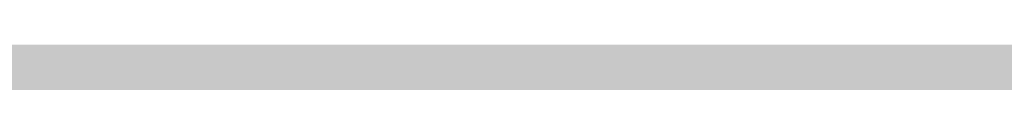
# Model space of a CAD drawing. Units: feet. Extents: x 3168 to 4724, y 827 to 1477.
# Tile 196 of 256: x 3316.07 to 3333.46, y 1098.34 to 1099. Entities that reach past the tile are written whole.
import ezdxf

# ---------------------------------------------------------------- set-up
doc = ezdxf.new("R2010")
doc.units = ezdxf.units.FT
doc.layers.add('A-ELEV', color=7, linetype='Continuous', lineweight=35)
doc.layers.add('A-ELEV-PATT', color=8, linetype='Continuous', lineweight=13)

msp = doc.modelspace()

# ---------------------------------------------------------------- hatches: boundary and pattern name
at = {"layer": 'A-ELEV-PATT'}
h = msp.add_hatch(color=256, dxfattribs=at)
h.dxf.hatch_style = 1
edge = h.paths.add_edge_path()
edge.add_ellipse((3552.906, 979.22), major_axis=(36.745, 0), ratio=0.484848, start_angle=0, end_angle=360)
edge = h.paths.add_edge_path()
edge.add_ellipse((3559.892, 929.252), major_axis=(36.745, 0), ratio=0.484848, start_angle=0, end_angle=360)
edge = h.paths.add_edge_path()
edge.add_line((3299.317, 1198.606), (3479.917, 1198.606))
edge.add_line((3479.917, 1198.606), (3479.917, 1209.869))
edge.add_spline(control_points=[(3479.917, 1209.869), (3464.301, 1209.869), (3448.686, 1209.869), (3410.949, 1209.869), (3388.828, 1209.869), (3355.647, 1209.869), (3344.586, 1209.869), (3327.996, 1209.869), (3322.466, 1209.869), (3314.17, 1209.869), (3311.405, 1209.869), (3307.257, 1209.869), (3305.875, 1209.869), (3303.801, 1209.869), (3303.11, 1209.869), (3302.073, 1209.869), (3301.727, 1209.869), (3301.209, 1209.869), (3301.036, 1209.869), (3300.777, 1209.869), (3300.69, 1209.869), (3300.561, 1209.869), (3300.517, 1209.869), (3300.453, 1209.869), (3300.431, 1209.869), (3300.399, 1209.869), (3300.388, 1209.869), (3300.366, 1209.869), (3300.346, 1209.869), (3300.346, 1209.869), (3300.346, 1209.869), (3300.343, 1209.869), (3300.341, 1209.869), (3300.338, 1209.869), (3300.337, 1209.869), (3300.334, 1209.869), (3300.332, 1209.869), (3300.326, 1209.869), (3300.321, 1209.869), (3300.311, 1209.869), (3300.306, 1209.869), (3300.291, 1209.869), (3300.28, 1209.869), (3300.232, 1209.869), (3300.195, 1209.869), (3299.951, 1209.871), (3299.745, 1209.874), (3299.437, 1209.883), (3299.334, 1209.887), (3299.181, 1209.893), (3299.13, 1209.895), (3298.652, 1209.917), (3298.229, 1209.946), (3297.602, 1210.002), (3297.393, 1210.023), (3297.083, 1210.058), (3296.979, 1210.07), (3296.293, 1210.155), (3295.718, 1210.243), (3294.869, 1210.399), (3294.588, 1210.454), (3294.169, 1210.543), (3294.03, 1210.574), (3291.707, 1211.101), (3289.654, 1211.813), (3285.776, 1213.564), (3283.951, 1214.603), (3280.512, 1216.98), (3278.897, 1218.318), (3276.38, 1220.829), (3275.416, 1221.918), (3274.039, 1223.708), (3273.581, 1224.35), (3273.143, 1225.016)], knot_values=[39.119033, 39.119033, 39.119033, 39.119033, 39.286353, 39.286353, 39.523379, 39.523379, 39.641892, 39.641892, 39.701148, 39.701148, 39.730777, 39.730777, 39.745591, 39.745591, 39.752998, 39.752998, 39.756701, 39.756701, 39.758553, 39.758553, 39.759479, 39.759479, 39.759942, 39.759942, 39.760173, 39.760173, 39.760289, 39.760289, 39.760405, 39.760405, 39.760463, 39.760463, 39.763389, 39.763389, 39.764851, 39.764851, 39.767304, 39.767304, 39.773825, 39.773825, 39.78057, 39.78057, 39.79477, 39.79477, 39.845194, 39.845194, 40.126715, 40.126715, 40.267476, 40.267476, 40.337856, 40.337856, 40.927023, 40.927023, 41.221606, 41.221606, 41.368898, 41.368898, 42.202622, 42.202622, 42.619485, 42.619485, 42.827916, 42.827916, 46.118323, 46.118323, 49.408731, 49.408731, 52.699139, 52.699139, 54.927489, 54.927489, 56.104228, 56.104228, 56.104228, 56.104228], weights=[1, 1, 1, 1, 1, 1, 1, 1, 1, 1, 1, 1, 1, 1, 1, 1, 1, 1, 1, 1, 1, 1, 1, 1, 1, 1, 1, 1, 1, 1, 1, 1, 1, 1, 1, 1, 1, 1, 1, 1, 1, 1, 1, 1, 1, 1, 1, 1, 1, 1, 1, 1, 1, 1, 1, 1, 1, 1, 1, 1, 1, 1, 1, 1, 1, 1, 1, 1, 1, 1, 1, 1, 1, 1], degree=3, periodic=0)
edge.add_line((3273.143, 1225.016), (3273.143, 1099.016))
edge.add_line((3273.143, 1099.016), (3299.317, 1099.016))
edge.add_line((3299.317, 1099.016), (3299.317, 1198.606))
edge = h.paths.add_edge_path()
edge.add_line((3304.758, 1324.158), (3479.917, 1324.158))
edge.add_line((3479.917, 1324.158), (3479.917, 1335.715))
edge.add_line((3479.917, 1335.715), (3269.162, 1335.715))
edge.add_spline(control_points=[(3269.162, 1335.715), (3264.024, 1335.715), (3258.364, 1328.958), (3259.264, 1323.9)], knot_values=[0, 0, 0, 0, 15.412191, 15.412191, 15.412191, 15.412191], degree=3, periodic=0)
edge.add_line((3259.264, 1323.9), (3265.517, 1288.769))
edge.add_line((3265.517, 1288.769), (3275.265, 1261.546))
edge.add_line((3275.265, 1261.546), (3304.758, 1261.546))
edge.add_line((3304.758, 1261.546), (3304.758, 1324.158))
h = msp.add_hatch(color=256, dxfattribs=at)
h.dxf.hatch_style = 1
h.paths.add_polyline_path([(3384.525, 1099.016), (3335.029, 1099.016), (3299.317, 1099.016), (3273.143, 1099.016), (3217.565, 1099.016), (3168.069, 827.116), (3335.029, 827.116)])

# ---------------------------------------------------------------- linework, layer by layer
at = {"layer": 'A-ELEV'}
msp.add_open_spline([(3808.52, 1099.016), (3808.52, 1141.413), (3808.52, 1183.81), (3808.52, 1226.635), (3808.52, 1227.064), (3808.52, 1227.492), (3811.492, 1248.995), (3814.464, 1270.498), (3817.465, 1292.218), (3817.495, 1292.435), (3817.525, 1292.652), (3817.573, 1310.107), (3817.62, 1327.562), (3817.668, 1345.016), (3817.668, 1345.458), (3817.668, 1345.9), (3817.668, 1346.456), (3817.668, 1346.571), (3817.668, 1346.753), (3817.668, 1346.82), (3817.668, 1346.935), (3817.668, 1346.982), (3817.668, 1347.039), (3817.668, 1347.047), (3817.668, 1347.074), (3817.668, 1347.059), (3817.668, 1347.062), (3817.668, 1347.063), (3817.668, 1347.066), (3817.668, 1347.068), (3817.668, 1347.075), (3817.668, 1347.079), (3817.668, 1347.093), (3817.668, 1347.102), (3817.668, 1347.129), (3817.668, 1347.147), (3817.667, 1347.2), (3817.667, 1347.236), (3817.666, 1347.343), (3817.665, 1347.415), (3817.661, 1347.628), (3817.657, 1347.77), (3817.64, 1348.192), (3817.624, 1348.472), (3817.559, 1349.3), (3817.496, 1349.841), (3817.255, 1351.424), (3817.026, 1352.429), (3816.307, 1354.889), (3815.744, 1356.269), (3814.464, 1358.819), (3813.746, 1359.991), (3812.196, 1362.172), (3811.362, 1363.182), (3809.589, 1365.069), (3808.649, 1365.946), (3806.654, 1367.58), (3805.6, 1368.336), (3803.353, 1369.722), (3802.161, 1370.352), (3799.601, 1371.454), (3798.233, 1371.925), (3795.28, 1372.635), (3793.693, 1372.872), (3791.869, 1372.926), (3791.741, 1372.929), (3791.353, 1372.934), (3791.093, 1372.933), (3790.304, 1372.915), (3789.77, 1372.884), (3789.209, 1372.83), (3789.191, 1372.828), (3789.135, 1372.823), (3789.098, 1372.819), (3789.048, 1372.814), (3789.036, 1372.813), (3789, 1372.809), (3788.976, 1372.806), (3788.949, 1372.803), (3788.947, 1372.803), (3788.943, 1372.803), (3788.941, 1372.802), (3788.939, 1372.802), (3788.938, 1372.802), (3788.935, 1372.802), (3788.868, 1372.794), (3788.757, 1372.782), (3788.702, 1372.776), (3788.536, 1372.758), (3788.425, 1372.746), (3788.093, 1372.709), (3787.872, 1372.685), (3787.208, 1372.612), (3786.765, 1372.563), (3785.437, 1372.417), (3784.551, 1372.32), (3781.895, 1372.027), (3780.125, 1371.833), (3774.813, 1371.248), (3771.271, 1370.859), (3760.647, 1369.69), (3753.564, 1368.911), (3732.316, 1366.573), (3718.15, 1365.015), (3694.007, 1362.359), (3684.029, 1361.262), (3674.051, 1360.164), (3664.601, 1360.164), (3655.151, 1360.164), (3626.801, 1360.164), (3607.901, 1360.164), (3551.202, 1360.164), (3513.402, 1360.164), (3467.725, 1360.164), (3459.848, 1360.164), (3436.215, 1360.164), (3420.46, 1360.164), (3373.194, 1360.164), (3341.684, 1360.164), (3302.848, 1360.164), (3295.523, 1360.164), (3286.038, 1360.164), (3283.879, 1360.164), (3277.403, 1360.164), (3273.085, 1360.164), (3267.733, 1360.164), (3266.699, 1360.164), (3263.597, 1360.164), (3261.528, 1360.164), (3259.237, 1360.164), (3259.014, 1360.164), (3258.344, 1360.164), (3257.897, 1360.164), (3257.431, 1360.164), (3257.411, 1360.164), (3257.371, 1360.164), (3257.375, 1360.164), (3257.375, 1360.164), (3257.374, 1360.164), (3257.372, 1360.164), (3257.371, 1360.164), (3257.367, 1360.164), (3257.364, 1360.164), (3257.356, 1360.164), (3257.351, 1360.164), (3257.335, 1360.164), (3257.324, 1360.164), (3257.293, 1360.164), (3257.272, 1360.164), (3257.208, 1360.163), (3257.166, 1360.163), (3257.04, 1360.161), (3256.956, 1360.16), (3256.706, 1360.153), (3256.539, 1360.147), (3256.044, 1360.122), (3255.717, 1360.097), (3254.752, 1360), (3254.128, 1359.907), (3252.18, 1359.525), (3250.942, 1359.144), (3248.67, 1358.243), (3247.636, 1357.724), (3245.733, 1356.603), (3244.863, 1356.002), (3243.253, 1354.743), (3242.512, 1354.085), (3240.751, 1352.345), (3239.801, 1351.23), (3238.088, 1348.872), (3237.325, 1347.63), (3235.983, 1344.972), (3235.402, 1343.555), (3234.591, 1340.815), (3234.311, 1339.544), (3233.976, 1336.803), (3233.922, 1335.331), (3234.149, 1332.591), (3234.35, 1331.367), (3234.72, 1329.999), (3234.752, 1329.883), (3234.854, 1329.535), (3234.926, 1329.302), (3235.025, 1329.003), (3235.047, 1328.937), (3235.078, 1328.847), (3235.086, 1328.823), (3235.111, 1328.751), (3235.128, 1328.703), (3235.148, 1328.646), (3235.151, 1328.638), (3235.156, 1328.624), (3235.158, 1328.618), (3235.16, 1328.612), (3235.166, 1328.597), (3235.18, 1328.556), (3235.19, 1328.528), (3235.221, 1328.443), (3235.241, 1328.386), (3235.302, 1328.216), (3235.343, 1328.102), (3235.465, 1327.762), (3235.546, 1327.535), (3235.79, 1326.853), (3235.953, 1326.399), (3236.44, 1325.037), (3236.766, 1324.128), (3237.741, 1321.403), (3238.392, 1319.587), (3240.344, 1314.137), (3241.645, 1310.504), (3245.548, 1299.604), (3248.15, 1292.337), (3255.956, 1270.537), (3261.16, 1256.004), (3267.388, 1238.612), (3268.411, 1235.753), (3269.51, 1232.684), (3269.586, 1232.474), (3269.707, 1232.136), (3269.752, 1232.008), (3269.827, 1231.799), (3269.856, 1231.718), (3269.906, 1231.578), (3269.927, 1231.52), (3269.972, 1231.393), (3269.997, 1231.325), (3270.027, 1231.243), (3270.032, 1231.228), (3270.04, 1231.204), (3270.039, 1231.207), (3270.039, 1231.207), (3270.039, 1231.206), (3270.04, 1231.206), (3270.04, 1231.205), (3270.04, 1231.204), (3270.04, 1231.204), (3270.041, 1231.201), (3270.042, 1231.2), (3270.043, 1231.195), (3270.045, 1231.192), (3270.048, 1231.183), (3270.05, 1231.177), (3270.056, 1231.159), (3270.061, 1231.147), (3270.074, 1231.111), (3270.083, 1231.087), (3270.109, 1231.014), (3270.127, 1230.966), (3270.18, 1230.822), (3270.216, 1230.727), (3270.325, 1230.442), (3270.4, 1230.253), (3270.629, 1229.691), (3270.789, 1229.324), (3271.286, 1228.238), (3271.643, 1227.54), (3272.776, 1225.515), (3273.614, 1224.261), (3275.416, 1221.918), (3276.38, 1220.829), (3278.897, 1218.318), (3280.512, 1216.98), (3283.951, 1214.603), (3285.776, 1213.564), (3289.654, 1211.813), (3291.707, 1211.101), (3294.03, 1210.574), (3294.169, 1210.543), (3294.588, 1210.454), (3294.869, 1210.399), (3295.718, 1210.243), (3296.293, 1210.155), (3296.979, 1210.07), (3297.083, 1210.058), (3297.393, 1210.023), (3297.602, 1210.002), (3298.229, 1209.946), (3298.652, 1209.917), (3299.13, 1209.895), (3299.181, 1209.893), (3299.334, 1209.887), (3299.437, 1209.883), (3299.745, 1209.874), (3299.951, 1209.871), (3300.195, 1209.869), (3300.232, 1209.869), (3300.28, 1209.869), (3300.291, 1209.869), (3300.306, 1209.869), (3300.311, 1209.869), (3300.321, 1209.869), (3300.326, 1209.869), (3300.332, 1209.869), (3300.334, 1209.869), (3300.337, 1209.869), (3300.338, 1209.869), (3300.341, 1209.869), (3300.343, 1209.869), (3300.346, 1209.869), (3300.346, 1209.869), (3300.346, 1209.869), (3300.366, 1209.869), (3300.388, 1209.869), (3300.399, 1209.869), (3300.431, 1209.869), (3300.453, 1209.869), (3300.517, 1209.869), (3300.561, 1209.869), (3300.69, 1209.869), (3300.777, 1209.869), (3301.036, 1209.869), (3301.209, 1209.869), (3301.727, 1209.869), (3302.073, 1209.869), (3303.11, 1209.869), (3303.801, 1209.869), (3305.875, 1209.869), (3307.257, 1209.869), (3311.405, 1209.869), (3314.17, 1209.869), (3322.466, 1209.869), (3327.996, 1209.869), (3344.586, 1209.869), (3355.647, 1209.869), (3388.828, 1209.869), (3410.949, 1209.869), (3477.312, 1209.869), (3521.554, 1209.869), (3566.836, 1209.869), (3567.877, 1209.869), (3570.999, 1209.869), (3573.08, 1209.869), (3575.781, 1209.869), (3576.401, 1209.869), (3577.296, 1209.869), (3577.571, 1209.869), (3578.397, 1209.869), (3578.948, 1209.869), (3579.756, 1209.869), (3580.015, 1209.869), (3580.343, 1209.869), (3580.327, 1209.869), (3580.327, 1209.869), (3580.327, 1209.869), (3580.328, 1209.869), (3580.328, 1209.869), (3580.329, 1209.869), (3580.33, 1209.869), (3580.331, 1209.869), (3580.333, 1209.869), (3580.336, 1209.869), (3580.339, 1209.869), (3580.346, 1209.869), (3580.351, 1209.869), (3580.366, 1209.869), (3580.375, 1209.869), (3580.405, 1209.868), (3580.424, 1209.868), (3580.483, 1209.868), (3580.522, 1209.868), (3580.64, 1209.867), (3580.719, 1209.865), (3580.956, 1209.861), (3581.115, 1209.856), (3581.594, 1209.837), (3581.916, 1209.818), (3582.89, 1209.742), (3583.548, 1209.666), (3585.532, 1209.361), (3586.867, 1209.054), (3589.472, 1208.252), (3590.74, 1207.758), (3591.995, 1207.159), (3592.058, 1207.129), (3592.244, 1207.038), (3592.368, 1206.977), (3592.735, 1206.79), (3592.977, 1206.663), (3593.245, 1206.516), (3593.275, 1206.5), (3593.365, 1206.45), (3593.425, 1206.416), (3593.604, 1206.315), (3593.723, 1206.247), (3593.857, 1206.168), (3593.874, 1206.158), (3593.926, 1206.128), (3593.96, 1206.108), (3594.062, 1206.047), (3594.13, 1206.006), (3594.208, 1205.958), (3594.22, 1205.951), (3594.253, 1205.931), (3594.276, 1205.917), (3594.343, 1205.876), (3594.388, 1205.848), (3594.434, 1205.819), (3594.435, 1205.818), (3594.44, 1205.815), (3594.443, 1205.813), (3594.447, 1205.811), (3594.448, 1205.81), (3594.449, 1205.81), (3594.449, 1205.809), (3594.45, 1205.809), (3594.45, 1205.808), (3594.451, 1205.808), (3594.467, 1205.798), (3594.493, 1205.782), (3594.506, 1205.774), (3594.545, 1205.749), (3594.571, 1205.733), (3594.648, 1205.684), (3594.7, 1205.652), (3594.855, 1205.555), (3594.959, 1205.49), (3595.269, 1205.295), (3595.476, 1205.166), (3596.097, 1204.776), (3596.511, 1204.517), (3597.753, 1203.739), (3598.581, 1203.22), (3601.064, 1201.664), (3602.72, 1200.626), (3607.687, 1197.513), (3610.998, 1195.438), (3620.932, 1189.212), (3627.555, 1185.061), (3647.423, 1172.61), (3660.668, 1164.309), (3700.403, 1139.405), (3726.894, 1122.803), (3757.206, 1103.806), (3761.027, 1101.411), (3764.848, 1099.016), (3745.328, 1099.016), (3725.808, 1099.016), (3706.288, 1099.016), (3706.288, 1108.453), (3706.288, 1117.89), (3706.288, 1127.327), (3710.751, 1127.327), (3715.213, 1127.327), (3719.676, 1127.327)], degree=3, knots=[0, 0, 0, 0, 0.982037, 0.982037, 0.991957, 0.991957, 0.991957, 1.966522, 1.966522, 1.976367, 1.976367, 1.976367, 2.976367, 2.976367, 2.976367, 3.00169, 3.00169, 3.008272, 3.008272, 3.012129, 3.012129, 3.014851, 3.014851, 3.015353, 3.015353, 3.016359, 3.016359, 3.017365, 3.017365, 3.019376, 3.019376, 3.023398, 3.023398, 3.031442, 3.031442, 3.047531, 3.047531, 3.079708, 3.079708, 3.144063, 3.144063, 3.272772, 3.272772, 3.53019, 3.53019, 4.045026, 4.045026, 5.074698, 5.074698, 6.700878, 6.700878, 8.327058, 8.327058, 9.953238, 9.953238, 11.579418, 11.579418, 13.205598, 13.205598, 14.831778, 14.831778, 16.457958, 16.457958, 18.084138, 18.084138, 18.206872, 18.206872, 18.45234, 18.45234, 18.943275, 18.943275, 18.960093, 18.960093, 18.993729, 18.993729, 19.00461, 19.00461, 19.026374, 19.026374, 19.028737, 19.028737, 19.03018, 19.03018, 19.030897, 19.030897, 19.032332, 19.032332, 19.033766, 19.033766, 19.036636, 19.036636, 19.042374, 19.042374, 19.053851, 19.053851, 19.076805, 19.076805, 19.122714, 19.122714, 19.21453, 19.21453, 19.398163, 19.398163, 19.765429, 19.765429, 20.024128, 20.024128, 20.024128, 20.092031, 20.092031, 20.227836, 20.227836, 20.499446, 20.499446, 20.556051, 20.556051, 20.66926, 20.66926, 20.895678, 20.895678, 20.948316, 20.948316, 20.963829, 20.963829, 20.994855, 20.994855, 21.002285, 21.002285, 21.017146, 21.017146, 21.01875, 21.01875, 21.021959, 21.021959, 21.022102, 21.022102, 21.022249, 21.022249, 21.022708, 21.022708, 21.023627, 21.023627, 21.025464, 21.025464, 21.029138, 21.029138, 21.036486, 21.036486, 21.051183, 21.051183, 21.080575, 21.080575, 21.139361, 21.139361, 21.256932, 21.256932, 21.492073, 21.492073, 21.962356, 21.962356, 23.01002, 23.01002, 24.057684, 24.057684, 25.105348, 25.105348, 26.153011, 26.153011, 27.776787, 27.776787, 29.400562, 29.400562, 31.024337, 31.024337, 32.278801, 32.278801, 33.533265, 33.533265, 34.467568, 34.467568, 34.553971, 34.553971, 34.726776, 34.726776, 34.775309, 34.775309, 34.793079, 34.793079, 34.82862, 34.82862, 34.834979, 34.834979, 34.839039, 34.839039, 34.839411, 34.839411, 34.840285, 34.840285, 34.842034, 34.842034, 34.845531, 34.845531, 34.852525, 34.852525, 34.866512, 34.866512, 34.894488, 34.894488, 34.950439, 34.950439, 35.062342, 35.062342, 35.286147, 35.286147, 35.733758, 35.733758, 35.821815, 35.821815, 35.828283, 35.828283, 35.832225, 35.832225, 35.834724, 35.834724, 35.836521, 35.836521, 35.838617, 35.838617, 35.839073, 35.839073, 35.839345, 35.839345, 35.839617, 35.839617, 35.840161, 35.840161, 35.841249, 35.841249, 35.843425, 35.843425, 35.847778, 35.847778, 35.856482, 35.856482, 35.873891, 35.873891, 35.908709, 35.908709, 35.978345, 35.978345, 36.117617, 36.117617, 36.396161, 36.396161, 36.953248, 36.953248, 38.067423, 38.067423, 40.295772, 40.295772, 42.524122, 42.524122, 45.81453, 45.81453, 49.104937, 49.104937, 52.395345, 52.395345, 52.603776, 52.603776, 53.020639, 53.020639, 53.854363, 53.854363, 54.001655, 54.001655, 54.296238, 54.296238, 54.885405, 54.885405, 54.955785, 54.955785, 55.096546, 55.096546, 55.378067, 55.378067, 55.42849, 55.42849, 55.442691, 55.442691, 55.449436, 55.449436, 55.455957, 55.455957, 55.458409, 55.458409, 55.459872, 55.459872, 55.462798, 55.462798, 55.462856, 55.462856, 55.462972, 55.462972, 55.463088, 55.463088, 55.463319, 55.463319, 55.463782, 55.463782, 55.464708, 55.464708, 55.46656, 55.46656, 55.470263, 55.470263, 55.47767, 55.47767, 55.492484, 55.492484, 55.522112, 55.522112, 55.581369, 55.581369, 55.699882, 55.699882, 55.936907, 55.936907, 56.410959, 56.410959, 56.42211, 56.42211, 56.444413, 56.444413, 56.451051, 56.451051, 56.454001, 56.454001, 56.459901, 56.459901, 56.462666, 56.462666, 56.463418, 56.463418, 56.464171, 56.464171, 56.465675, 56.465675, 56.468684, 56.468684, 56.474702, 56.474702, 56.486738, 56.486738, 56.51081, 56.51081, 56.558955, 56.558955, 56.655243, 56.655243, 56.847821, 56.847821, 57.232975, 57.232975, 58.003284, 58.003284, 59.543901, 59.543901, 62.625137, 62.625137, 68.787607, 68.787607, 74.950078, 74.950078, 75.27336, 75.27336, 75.919923, 75.919923, 77.213051, 77.213051, 77.377769, 77.377769, 77.707206, 77.707206, 78.366079, 78.366079, 78.462532, 78.462532, 78.655436, 78.655436, 79.041245, 79.041245, 79.105735, 79.105735, 79.234714, 79.234714, 79.492672, 79.492672, 79.502197, 79.502197, 79.521249, 79.521249, 79.523534, 79.523534, 79.528103, 79.528103, 79.528682, 79.528682, 79.528885, 79.528885, 79.529089, 79.529089, 79.529495, 79.529495, 79.530308, 79.530308, 79.531935, 79.531935, 79.535187, 79.535187, 79.541693, 79.541693, 79.554704, 79.554704, 79.580725, 79.580725, 79.632769, 79.632769, 79.736856, 79.736856, 79.94503, 79.94503, 80.361377, 80.361377, 80.421435, 80.421435, 80.421435, 81.421435, 81.421435, 81.421435, 82.421435, 82.421435, 82.421435, 83.421435, 83.421435, 83.421435, 83.421435], dxfattribs=at)

doc.saveas('drawing.dxf')
